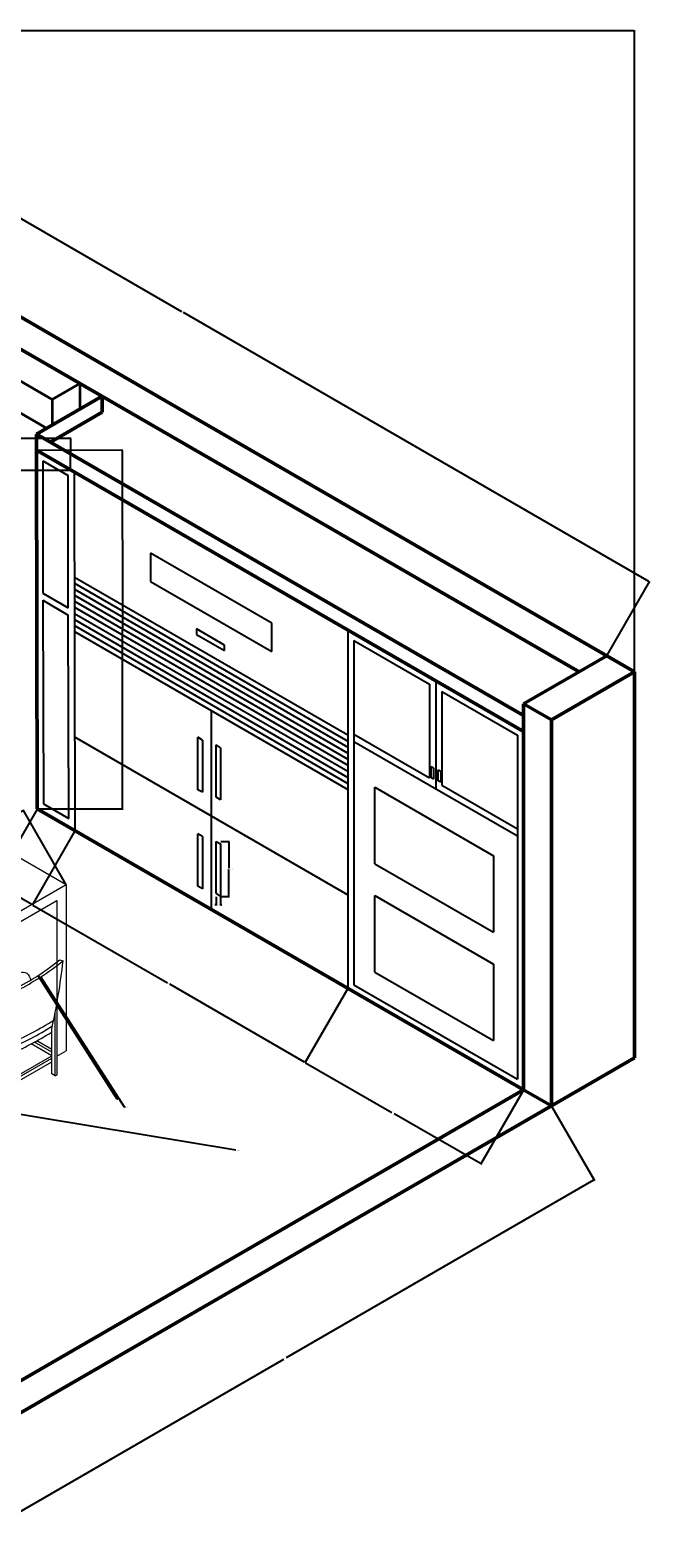
# Model space of a CAD drawing. Units: inches. Extents: x 4150 to 4636, y 2169 to 2592.
# Tile 8 of 8: x 4462 to 4636, y 2169 to 2592. Entities that reach past the tile are written whole.
import ezdxf

# ---------------------------------------------------------------- set-up
doc = ezdxf.new("R2010")
doc.units = ezdxf.units.IN
for name, color, linetype, lineweight in [('A-ANNO-DIMS', 2, 'Continuous', 18), ('A-EQPM', 6, 'Continuous', 25), ('A-FURN', 8, 'Continuous', 18), ('A-WALL', 7, 'Continuous', 50), ('S-BEAM', 1, 'Continuous', 35)]:
    doc.layers.add(name, color=color, linetype=linetype, lineweight=lineweight)
doc.styles.get("Standard").update_dxf_attribs({"font": 'arial.ttf'})
doc.dimstyles.get("Standard").update_dxf_attribs({"dimtxt": 0.18, "dimasz": 0.18, "dimexe": 0.18, "dimexo": 0.0625, "dimgap": 0.09, "dimtad": 0, "dimtih": 1, "dimtoh": 1, "dimdec": 4, "dimzin": 0, "dimdsep": 46, "dimtxsty": 'Standard', "dimcen": 0.09, "dimadec": 0, "dimazin": 0, "dimtfac": 1, "dimtdec": 4, "dimtofl": 0, "dimtmove": 0, "dimatfit": 3, "dimfxl": 1, "dimtolj": 1, "dimtzin": 0, "dimarcsym": 0})

# ---------------------------------------------------------------- blocks, each defined once
blk = doc.blocks.new('CHAIR')
for p, q in [((4460.61, 2323.17), (4462.07, 2322.64)), ((4458.4, 2267.81), (4458.4, 2298.32)), ((4459.26, 2268.31), (4459.26, 2302.96)), ((4419.13, 2296.33), (4418.72, 2294.28)), ((4434.61, 2281.77), (4418.72, 2294.28)), ((4418.72, 2294.28), (4418.72, 2263.74)), ((4435.02, 2283.82), (4419.13, 2296.33)), ((4419.58, 2264.24), (4419.58, 2293.6)), ((4421.31, 2292.24), (4421.31, 2265.24)), ((4436.24, 2283.27), (4435.02, 2283.82)), ((4456.67, 2279.13), (4448.46, 2283.88)), ((4456.67, 2280.34), (4449.53, 2284.46)), ((4456.67, 2268.81), (4456.67, 2290.03)), ((4421.31, 2274.06), (4434.6, 2281.73)), ((4421.31, 2272.85), (4434.31, 2280.36)), ((4421.31, 2271.17), (4433.9, 2278.43)), ((4435.2, 2254.23), (4435.2, 2278.19)), ((4436.06, 2254.73), (4436.06, 2282.33)), ((4436.06, 2265.55), (4456.67, 2277.45)), ((4456.67, 2277.45), (4446.94, 2283.07)), ((4433.46, 2267.05), (4421.31, 2274.06)), ((4433.46, 2265.84), (4421.31, 2272.85)), ((4433.46, 2264.15), (4421.31, 2271.17)), ((4433.46, 2255.23), (4433.46, 2276.44)), ((4436.06, 2264.34), (4456.67, 2276.24)), ((4436.06, 2262.66), (4456.67, 2274.56)), ((4418.72, 2263.74), (4419.58, 2264.24)), ((4419.58, 2264.24), (4421.31, 2265.24)), ((4458.4, 2267.81), (4456.67, 2268.81)), ((4458.4, 2267.81), (4459.26, 2268.31)), ((4435.2, 2254.23), (4433.46, 2255.23)), ((4435.2, 2254.23), (4436.06, 2254.73))]:
    blk.add_line(p, q)
for centre, radius, start, end in [((4387.22, 2413.69), 116.53, 296.3285, 309.03474), ((4384.96, 2418.26), 122.84, 296.66524, 308.88253), ((4169.51, 2354.34), 294.27, 347.37626, 353.81529), ((4146.35, 2340.95), 294.27, 347.33851, 353.81529), ((4147.53, 2340.19), 294.27, 347.83822, 353.81529), ((4388.03, 2399.21), 127.8, 292.07351, 302.67553), ((4388.03, 2401.62), 127.8, 292.16404, 302.99309), ((4387.7, 2396.31), 127.8, 292.23455, 302.66255)]:
    blk.add_arc(centre, radius, start, end)
blk.add_open_spline([(4419.13, 2296.33), (4419.73, 2299.09), (4421.22, 2306.03), (4435.02, 2305.47), (4437.67, 2317.36), (4445.4, 2317.24), (4446.24, 2314.8), (4446.7, 2313.47)], degree=3, knots=[0, 0, 0, 0, 7.695976, 19.302291, 31.993754, 35.157842, 38.967805, 38.967805, 38.967805, 38.967805])
blk = doc.blocks.new('FRIDGE-HANDLE')
for p, q in [((0, 0.81), (0, 15.46)), ((0, 15.46), (1.26, 14.74)), ((1.26, 14.74), (1.26, 0)), ((0, 0.81), (1.26, 0))]:
    blk.add_line(p, q)
blk = doc.blocks.new('*D24')
at = {"layer": 'A-ANNO-DIMS', "color": 0, "lineweight": -2, "transparency": 16777216}
for p, q in [((4515.27, 2364.38), (4517.7, 2364.38)), ((4517.52, 2364.2), (4517.52, 2356.83)), ((4517.52, 2349.1), (4517.52, 2356.46)), ((4515.27, 2348.92), (4517.7, 2348.92))]:
    blk.add_line(p, q, dxfattribs=at)
at = {"layer": 'A-ANNO-DIMS', "color": 0, "transparency": 16777216}
for points in [[(4517.49, 2364.2), (4517.55, 2364.2), (4517.52, 2364.38)], [(4517.49, 2349.1), (4517.55, 2349.1), (4517.52, 2348.92)]]:
    blk.add_solid(points, dxfattribs=at)
at = {"layer": 'Defpoints', "color": 0, "transparency": 16777216}
for p in [(4515.2, 2364.38), (4517.52, 2364.38), (4515.2, 2348.92)]:
    blk.add_point(p, dxfattribs=at)
at = {"layer": 'A-ANNO-DIMS', "color": 0, "transparency": 16777216, "insert": (4517.52, 2356.65), "char_height": 0.18, "attachment_point": 5}
blk.add_mtext('\\A1;FRIDGE HANDLE 15 TYP.', dxfattribs=at)
blk = doc.blocks.new('*D25')
at = {"layer": 'A-ANNO-DIMS', "color": 0, "lineweight": -2, "transparency": 16777216}
for p, q in [((4513.76, 2346.6), (4513.58, 2346.6)), ((4513.94, 2348.85), (4513.94, 2346.42)), ((4515.2, 2348.85), (4515.2, 2346.42)), ((4515.38, 2346.6), (4515.56, 2346.6))]:
    blk.add_line(p, q, dxfattribs=at)
at = {"layer": 'A-ANNO-DIMS', "color": 0, "transparency": 16777216}
for points in [[(4513.76, 2346.63), (4513.76, 2346.57), (4513.94, 2346.6)], [(4515.38, 2346.63), (4515.38, 2346.57), (4515.2, 2346.6)]]:
    blk.add_solid(points, dxfattribs=at)
at = {"layer": 'Defpoints', "color": 0, "transparency": 16777216}
for p in [(4513.94, 2348.92), (4515.2, 2348.92), (4515.2, 2346.6)]:
    blk.add_point(p, dxfattribs=at)
at = {"layer": 'A-ANNO-DIMS', "color": 0, "transparency": 16777216, "insert": (4514.57, 2346.6), "char_height": 0.18, "attachment_point": 5}
blk.add_mtext('\\A1;1 TYP.', dxfattribs=at)
blk = doc.blocks.new('*D36')
at = {"layer": 'A-ANNO-DIMS', "color": 0, "lineweight": -2, "transparency": 16777216}
for p, q in [((4174.28, 2460.03), (4174.28, 2592.15)), ((4174.46, 2591.97), (4402.51, 2591.97)), ((4631.36, 2591.97), (4403.31, 2591.97)), ((4631.54, 2412.03), (4631.54, 2592.15))]:
    blk.add_line(p, q, dxfattribs=at)
at = {"layer": 'A-ANNO-DIMS', "color": 0, "transparency": 16777216}
for points in [[(4174.46, 2592), (4174.46, 2591.94), (4174.28, 2591.97)], [(4631.36, 2592), (4631.36, 2591.94), (4631.54, 2591.97)]]:
    blk.add_solid(points, dxfattribs=at)
at = {"layer": 'Defpoints', "color": 0, "transparency": 16777216}
for p in [(4631.54, 2591.97), (4174.28, 2459.97), (4631.54, 2411.97)]:
    blk.add_point(p, dxfattribs=at)
at = {"layer": 'A-ANNO-DIMS', "color": 0, "transparency": 16777216, "insert": (4402.91, 2591.97), "char_height": 0.18, "attachment_point": 5}
blk.add_mtext('\\A1;457.3', dxfattribs=at)
blk = doc.blocks.new('*D39')
at = {"layer": 'A-ANNO-DIMS', "color": 0, "lineweight": -2, "transparency": 16777216}
for p, q in [((4608.19, 2290.05), (4620.25, 2269.16)), ((4620, 2269.23), (4533.6, 2219.34)), ((4446.56, 2169.09), (4532.97, 2218.98)), ((4434.43, 2189.73), (4446.49, 2168.84))]:
    blk.add_line(p, q, dxfattribs=at)
at = {"layer": 'A-ANNO-DIMS', "color": 0, "transparency": 16777216}
for points in [[(4619.99, 2269.25), (4620.02, 2269.2), (4620.16, 2269.32)], [(4446.54, 2169.11), (4446.57, 2169.06), (4446.4, 2169)]]:
    blk.add_solid(points, dxfattribs=at)
at = {"layer": 'Defpoints', "color": 0, "transparency": 16777216}
for p in [(4608.16, 2290.1), (4434.4, 2189.78), (4446.4, 2169)]:
    blk.add_point(p, dxfattribs=at)
at = {"layer": 'A-ANNO-DIMS', "color": 0, "transparency": 16777216, "insert": (4533.28, 2219.16), "char_height": 0.18, "attachment_point": 5}
blk.add_mtext('\\A1;200.64', dxfattribs=at)
blk = doc.blocks.new('*D43')
at = {"layer": 'A-ANNO-DIMS', "color": 0, "lineweight": -2, "transparency": 16777216}
for p, q in [((4361.37, 2568.02), (4373.43, 2588.91)), ((4373.5, 2588.66), (4504.26, 2513.17)), ((4635.59, 2437.34), (4504.83, 2512.83)), ((4623.78, 2416.52), (4635.84, 2437.41))]:
    blk.add_line(p, q, dxfattribs=at)
at = {"layer": 'A-ANNO-DIMS', "color": 0, "transparency": 16777216}
for points in [[(4373.51, 2588.69), (4373.48, 2588.63), (4373.34, 2588.75)], [(4635.61, 2437.37), (4635.58, 2437.31), (4635.75, 2437.25)]]:
    blk.add_solid(points, dxfattribs=at)
at = {"layer": 'Defpoints', "color": 0, "transparency": 16777216}
for p in [(4361.34, 2567.97), (4635.75, 2437.25), (4623.75, 2416.47)]:
    blk.add_point(p, dxfattribs=at)
at = {"layer": 'A-ANNO-DIMS', "color": 0, "transparency": 16777216, "insert": (4504.54, 2513), "char_height": 0.18, "attachment_point": 5}
blk.add_mtext('\\A1;303', dxfattribs=at)
blk = doc.blocks.new('*D46')
at = {"layer": 'A-ANNO-DIMS', "color": 0, "lineweight": -2, "transparency": 16777216}
for p, q in [((4449.11, 2477.6), (4473.23, 2477.6)), ((4473.05, 2477.42), (4473.05, 2473.29)), ((4473.05, 2468.78), (4473.05, 2472.92)), ((4449.11, 2468.6), (4473.23, 2468.6))]:
    blk.add_line(p, q, dxfattribs=at)
at = {"layer": 'A-ANNO-DIMS', "color": 0, "transparency": 16777216}
for points in [[(4473.02, 2477.42), (4473.08, 2477.42), (4473.05, 2477.6)], [(4473.02, 2468.78), (4473.08, 2468.78), (4473.05, 2468.6)]]:
    blk.add_solid(points, dxfattribs=at)
at = {"layer": 'Defpoints', "color": 0, "transparency": 16777216}
for p in [(4449.05, 2477.6), (4449.05, 2468.6), (4473.05, 2468.6)]:
    blk.add_point(p, dxfattribs=at)
at = {"layer": 'A-ANNO-DIMS', "color": 0, "transparency": 16777216, "insert": (4473.05, 2473.1), "char_height": 0.18, "attachment_point": 5}
blk.add_mtext('\\A1;9', dxfattribs=at)
blk = doc.blocks.new('*D62')
at = {"layer": 'A-ANNO-DIMS', "color": 0, "lineweight": -2, "transparency": 16777216}
for p, q in [((4463.66, 2373.46), (4451.6, 2352.57)), ((4474.29, 2367.32), (4462.23, 2346.43)), ((4451.85, 2352.64), (4456.69, 2349.84)), ((4462.17, 2346.68), (4457.32, 2349.48))]:
    blk.add_line(p, q, dxfattribs=at)
at = {"layer": 'A-ANNO-DIMS', "color": 0, "transparency": 16777216}
for points in [[(4451.86, 2352.66), (4451.83, 2352.61), (4451.69, 2352.73)], [(4462.18, 2346.7), (4462.15, 2346.65), (4462.32, 2346.59)]]:
    blk.add_solid(points, dxfattribs=at)
at = {"layer": 'Defpoints', "color": 0, "transparency": 16777216}
for p in [(4463.69, 2373.51), (4474.32, 2367.37), (4451.69, 2352.73)]:
    blk.add_point(p, dxfattribs=at)
at = {"layer": 'A-ANNO-DIMS', "color": 0, "transparency": 16777216, "insert": (4457.01, 2349.66), "char_height": 0.18, "attachment_point": 5}
blk.add_mtext('\\A1;12.278', dxfattribs=at)
blk = doc.blocks.new('*D63')
at = {"layer": 'A-ANNO-DIMS', "color": 0, "lineweight": -2, "transparency": 16777216}
for p, q in [((4474.29, 2367.32), (4462.23, 2346.43)), ((4462.48, 2346.5), (4500.33, 2324.65)), ((4538.8, 2302.43), (4500.96, 2324.28)), ((4550.93, 2323.07), (4538.87, 2302.19))]:
    blk.add_line(p, q, dxfattribs=at)
at = {"layer": 'A-ANNO-DIMS', "color": 0, "transparency": 16777216}
for points in [[(4462.49, 2346.52), (4462.46, 2346.47), (4462.32, 2346.59)], [(4538.82, 2302.46), (4538.79, 2302.41), (4538.96, 2302.34)]]:
    blk.add_solid(points, dxfattribs=at)
at = {"layer": 'Defpoints', "color": 0, "transparency": 16777216}
for p in [(4474.32, 2367.37), (4462.32, 2346.59), (4550.96, 2323.13)]:
    blk.add_point(p, dxfattribs=at)
at = {"layer": 'A-ANNO-DIMS', "color": 0, "transparency": 16777216, "insert": (4500.64, 2324.46), "char_height": 0.18, "attachment_point": 5}
blk.add_mtext('\\A1;88.5', dxfattribs=at)
blk = doc.blocks.new('*D64')
at = {"layer": 'A-ANNO-DIMS', "color": 0, "lineweight": -2, "transparency": 16777216}
for p, q in [((4550.93, 2323.07), (4538.87, 2302.19)), ((4539.11, 2302.25), (4563.35, 2288.26)), ((4600.33, 2294.55), (4588.27, 2273.66)), ((4588.21, 2273.91), (4563.98, 2287.9))]:
    blk.add_line(p, q, dxfattribs=at)
at = {"layer": 'A-ANNO-DIMS', "color": 0, "transparency": 16777216}
for points in [[(4539.13, 2302.28), (4539.1, 2302.23), (4538.96, 2302.34)], [(4588.22, 2273.93), (4588.19, 2273.88), (4588.36, 2273.82)]]:
    blk.add_solid(points, dxfattribs=at)
at = {"layer": 'Defpoints', "color": 0, "transparency": 16777216}
for p in [(4550.96, 2323.13), (4538.96, 2302.34), (4600.36, 2294.6)]:
    blk.add_point(p, dxfattribs=at)
at = {"layer": 'A-ANNO-DIMS', "color": 0, "transparency": 16777216, "insert": (4563.66, 2288.08), "char_height": 0.18, "attachment_point": 5}
blk.add_mtext('\\A1;57.05', dxfattribs=at)
blk = doc.blocks.new('*D65')
at = {"layer": 'A-ANNO-DIMS', "color": 0, "lineweight": -2, "transparency": 16777216}
for p, q in [((4463.58, 2474.23), (4487.7, 2474.28)), ((4487.52, 2474.1), (4487.6, 2424.1)), ((4487.69, 2373.73), (4487.6, 2423.73)), ((4463.75, 2373.51), (4487.87, 2373.55))]:
    blk.add_line(p, q, dxfattribs=at)
at = {"layer": 'A-ANNO-DIMS', "color": 0, "transparency": 16777216}
for points in [[(4487.55, 2474.1), (4487.49, 2474.1), (4487.52, 2474.28)], [(4487.72, 2373.73), (4487.66, 2373.73), (4487.69, 2373.55)]]:
    blk.add_solid(points, dxfattribs=at)
at = {"layer": 'Defpoints', "color": 0, "transparency": 16777216}
for p in [(4463.52, 2474.23), (4463.69, 2373.51), (4487.69, 2373.55)]:
    blk.add_point(p, dxfattribs=at)
at = {"layer": 'A-ANNO-DIMS', "color": 0, "transparency": 16777216, "insert": (4487.6, 2423.91), "char_height": 0.18, "attachment_point": 5}
blk.add_mtext('\\A1;100.72', dxfattribs=at)
blk = doc.blocks.new('*D67')
at = {"layer": 'A-ANNO-DIMS', "color": 0, "lineweight": -2, "transparency": 16777216}
for p, q in [((4459.63, 2373), (4418.44, 2349.22)), ((4471.75, 2352.36), (4459.7, 2373.25)), ((4376.8, 2325.18), (4418, 2348.96)), ((4388.62, 2304.36), (4376.56, 2325.25))]:
    blk.add_line(p, q, dxfattribs=at)
at = {"layer": 'A-ANNO-DIMS', "color": 0, "transparency": 16777216}
for points in [[(4459.62, 2373.03), (4459.65, 2372.98), (4459.79, 2373.09)], [(4376.79, 2325.21), (4376.82, 2325.16), (4376.65, 2325.09)]]:
    blk.add_solid(points, dxfattribs=at)
at = {"layer": 'Defpoints', "color": 0, "transparency": 16777216}
for p in [(4459.79, 2373.09), (4471.79, 2352.31), (4388.65, 2304.31)]:
    blk.add_point(p, dxfattribs=at)
at = {"layer": 'A-ANNO-DIMS', "color": 0, "transparency": 16777216, "insert": (4418.22, 2349.09), "char_height": 0.18, "attachment_point": 5}
blk.add_mtext('\\A1;96', dxfattribs=at)
blk = doc.blocks.new('*D75')
at = {"layer": 'A-ANNO-DIMS', "color": 0, "lineweight": -2, "transparency": 16777216}
for p, q in [((4245.64, 2323.02), (4245.82, 2323.02)), ((4245.73, 2322.93), (4245.73, 2323.11)), ((4519.53, 2277.67), (4417.03, 2294.65))]:
    blk.add_line(p, q, dxfattribs=at)
at = {"layer": 'A-ANNO-DIMS', "color": 0, "transparency": 16777216}
blk.add_solid([(4417.03, 2294.68), (4417.02, 2294.62), (4416.85, 2294.68)], dxfattribs=at)
at = {"layer": 'Defpoints', "color": 0, "transparency": 16777216}
for p in [(4245.73, 2323.02), (4416.85, 2294.68)]:
    blk.add_point(p, dxfattribs=at)
at = {"layer": 'A-ANNO-DIMS', "color": 0, "transparency": 16777216, "insert": (4520.08, 2277.67), "char_height": 0.18, "attachment_point": 5}
blk.add_mtext('\\A1;R173.46', dxfattribs=at)
blk = doc.blocks.new('*D77')
at = {"layer": 'A-ANNO-DIMS', "color": 0, "lineweight": -2, "transparency": 16777216}
for p, q in [((4425.39, 2387.21), (4425.57, 2387.21)), ((4425.48, 2387.12), (4425.48, 2387.3)), ((4488.19, 2289.8), (4464.77, 2326.18)), ((4488.37, 2289.8), (4488.19, 2289.8))]:
    blk.add_line(p, q, dxfattribs=at)
at = {"layer": 'A-ANNO-DIMS', "color": 0, "transparency": 16777216}
blk.add_solid([(4464.8, 2326.19), (4464.75, 2326.16), (4464.68, 2326.33)], dxfattribs=at)
at = {"layer": 'Defpoints', "color": 0, "transparency": 16777216}
for p in [(4425.48, 2387.21), (4464.68, 2326.33)]:
    blk.add_point(p, dxfattribs=at)
at = {"layer": 'A-ANNO-DIMS', "color": 0, "transparency": 16777216, "insert": (4488.84, 2289.8), "char_height": 0.18, "attachment_point": 5}
blk.add_mtext('\\A1;R72.41', dxfattribs=at)
blk = doc.blocks.new('*D78')
at = {"layer": 'A-ANNO-DIMS', "color": 0, "lineweight": -2, "transparency": 16777216}
for p, q in [((4426.72, 2384.51), (4426.9, 2384.51)), ((4426.81, 2384.42), (4426.81, 2384.6)), ((4486.16, 2292.01), (4464, 2326.55)), ((4486.34, 2292.01), (4486.16, 2292.01))]:
    blk.add_line(p, q, dxfattribs=at)
at = {"layer": 'A-ANNO-DIMS', "color": 0, "transparency": 16777216}
blk.add_solid([(4464.03, 2326.56), (4463.98, 2326.53), (4463.9, 2326.7)], dxfattribs=at)
at = {"layer": 'Defpoints', "color": 0, "transparency": 16777216}
for p in [(4426.81, 2384.51), (4463.9, 2326.7)]:
    blk.add_point(p, dxfattribs=at)
at = {"layer": 'A-ANNO-DIMS', "color": 0, "transparency": 16777216, "insert": (4486.82, 2292.01), "char_height": 0.18, "attachment_point": 5}
blk.add_mtext('\\A1;R68.69', dxfattribs=at)

msp = doc.modelspace()

# ---------------------------------------------------------------- linework, layer by layer
at = {"layer": 'A-EQPM'}
for p, q in [((4465.2501, 2471.2343), (4465.2501, 2434.0676)), ((4465.2501, 2471.2343), (4472.4192, 2467.0952)), ((4474.3231, 2367.372), (4474.1513, 2468.0952)), ((4474.1513, 2468.0952), (4550.9589, 2423.7503)), ((4472.4192, 2429.9285), (4472.4192, 2467.0952)), ((4529.5665, 2425.6516), (4495.5437, 2445.2946)), ((4495.5437, 2445.2946), (4495.5437, 2437.3101)), ((4474.1513, 2438.6014), (4550.9589, 2394.2565)), ((4465.2501, 2434.0676), (4472.4192, 2429.9285)), ((4474.1513, 2436.9011), (4550.9589, 2392.5562)), ((4474.1513, 2435.2008), (4550.9589, 2390.8559)), ((4495.5437, 2437.3101), (4529.5665, 2417.667)), ((4465.2501, 2432.0676), (4472.4192, 2427.9285)), ((4465.2501, 2432.0676), (4465.4213, 2374.9185)), ((4474.1513, 2433.5006), (4550.9589, 2389.1557)), ((4474.1513, 2431.8003), (4550.9589, 2387.4554)), ((4474.1513, 2430.1), (4550.9589, 2385.7551)), ((4472.5904, 2370.7794), (4472.4192, 2427.9285)), ((4474.1513, 2428.3997), (4550.9589, 2384.0548)), ((4474.1513, 2426.6995), (4550.9589, 2382.3545)), ((4529.5665, 2417.667), (4529.5665, 2425.6516)), ((4474.1513, 2424.9992), (4550.9589, 2380.6543)), ((4474.1513, 2423.2989), (4550.9589, 2378.954)), ((4516.3444, 2419.5139), (4508.4817, 2424.0535)), ((4508.4817, 2424.0535), (4508.4817, 2422.4819)), ((4508.4817, 2422.4819), (4516.3444, 2417.9424)), ((4550.9589, 2423.7503), (4550.9589, 2323.1264)), ((4516.3444, 2417.9424), (4516.3444, 2419.5139)), ((4552.691, 2420.7503), (4552.691, 2324.1264)), ((4552.691, 2420.7503), (4573.9296, 2408.4882)), ((4575.6617, 2409.4882), (4575.6617, 2379.1849)), ((4573.9296, 2408.4882), (4573.9296, 2382.1849)), ((4577.3937, 2406.4882), (4577.3937, 2380.1849)), ((4577.3937, 2406.4882), (4598.6324, 2394.226)), ((4512.5551, 2401.1264), (4512.5551, 2345.2988)), ((4474.1513, 2393.699), (4550.9589, 2349.3541)), ((4552.691, 2394.4471), (4573.9296, 2382.1849)), ((4552.691, 2392.4471), (4598.6324, 2365.9227)), ((4598.6324, 2394.226), (4598.6324, 2297.602)), ((4574.3544, 2382.2326), (4574.3544, 2385.3699)), ((4574.3544, 2385.3699), (4575.03, 2384.9798)), ((4575.03, 2384.9798), (4575.03, 2381.8426)), ((4576.3824, 2381.3704), (4576.3824, 2384.5077)), ((4576.3824, 2384.5077), (4577.0579, 2384.1177)), ((4577.0579, 2384.1177), (4577.0579, 2380.9804)), ((4558.5181, 2358.0987), (4558.5181, 2379.5967)), ((4558.5181, 2379.5967), (4591.8494, 2360.3529)), ((4575.03, 2381.8426), (4574.3544, 2382.2326)), ((4577.0579, 2380.9804), (4576.3824, 2381.3704)), ((4577.3937, 2380.1849), (4598.6324, 2367.9227)), ((4465.4213, 2374.9185), (4472.5904, 2370.7794)), ((4463.513, 2373.6133), (4474.1462, 2367.4742)), ((4558.5181, 2358.0987), (4591.8494, 2338.8549)), ((4591.8494, 2360.3529), (4591.8494, 2338.8549)), ((4558.5181, 2327.6892), (4558.5181, 2349.1873)), ((4558.5181, 2349.1873), (4591.8494, 2329.9434)), ((4591.8494, 2329.9434), (4591.8494, 2308.4454)), ((4552.691, 2324.1264), (4598.6324, 2297.602)), ((4558.5181, 2327.6892), (4591.8494, 2308.4454)), ((4552.691, 2322.1264), (4598.6324, 2295.602))]:
    msp.add_line(p, q, dxfattribs=at)
at = {"layer": 'A-FURN'}
for p, q in [((4432.8151, 2374.8064), (4471.7862, 2352.3064)), ((4388.6478, 2304.3064), (4471.7862, 2352.3064)), ((4471.7862, 2352.3064), (4471.7862, 2305.5436)), ((4391.2458, 2302.8064), (4469.1881, 2347.8064)), ((4469.1881, 2347.8064), (4469.1881, 2304.0436)), ((4469.1881, 2304.0436), (4471.7862, 2305.5436))]:
    msp.add_line(p, q, dxfattribs=at)
at = {"layer": 'A-WALL'}
for p, q in [((4361.3415, 2567.9652), (4506.8337, 2483.9652)), ((4361.3415, 2558.9652), (4615.9529, 2411.9652)), ((4463.5181, 2478.7343), (4481.9117, 2489.3539)), ((4481.9117, 2489.3539), (4481.9117, 2484.8539)), ((4481.9117, 2484.8539), (4467.4152, 2476.4843)), ((4506.8337, 2483.9652), (4631.5414, 2411.9652)), ((4463.5181, 2474.2343), (4463.5181, 2478.7343)), ((4463.5181, 2478.7343), (4600.3645, 2399.726)), ((4463.5181, 2474.2343), (4600.3645, 2395.226)), ((4463.5181, 2474.2343), (4463.6899, 2373.5111)), ((4552.691, 2422.7503), (4600.3645, 2395.226)), ((4600.3645, 2402.9652), (4623.7472, 2416.4652)), ((4631.5414, 2411.9652), (4608.1587, 2398.4652)), ((4631.5414, 2411.9652), (4631.5414, 2303.602)), ((4608.1587, 2398.4652), (4600.3645, 2402.9652)), ((4600.3645, 2402.9652), (4600.3645, 2294.602)), ((4600.3645, 2402.9652), (4608.1587, 2398.4652)), ((4608.1587, 2398.4652), (4608.1587, 2290.102)), ((4600.3645, 2294.602), (4463.6899, 2373.5111)), ((4434.4021, 2189.7836), (4631.5414, 2303.602)), ((4434.204, 2198.6692), (4600.3645, 2294.602)), ((4608.1587, 2290.102), (4600.3645, 2294.602))]:
    msp.add_line(p, q, dxfattribs=at)
at = {"layer": 'S-BEAM'}
for p, q in [((4353.5472, 2554.4652), (4467.8626, 2488.4652)), ((4353.5472, 2545.4652), (4466.3233, 2480.3539)), ((4475.6568, 2492.9652), (4467.8626, 2488.4652)), ((4475.6568, 2492.9652), (4475.6568, 2485.7426)), ((4467.8626, 2488.4652), (4467.8626, 2481.2426))]:
    msp.add_line(p, q, dxfattribs=at)

# ---------------------------------------------------------------- block references
at = {"layer": 'A-EQPM', "rotation": 180.0247430787337}
for p in [(4510.1055, 2393.6222), (4515.1991, 2391.4957), (4510.1055, 2366.5481)]:
    msp.add_blockref('FRIDGE-HANDLE', p, dxfattribs=at)
at = {"layer": 'A-EQPM'}
msp.add_blockref('FRIDGE-HANDLE', (4513.945, 2348.915), dxfattribs=at)
at = {"layer": 'A-FURN', "xscale": 0.5894434727893052, "yscale": 0.5894434727893052, "zscale": 0.5894434727893052}
msp.add_blockref('CHAIR', (1840.7944, 961.7822), dxfattribs=at)

# ---------------------------------------------------------------- dimensions: what is measured, and where the dimension line sits
at = {"layer": 'A-ANNO-DIMS'}
dim = msp.add_linear_dim(base=(4631.5414, 2591.9652), p1=(4174.28, 2459.9652), p2=(4631.5414, 2411.9652), dimstyle='Standard', override={"dimdec": 1, "dimlfac": 1, "dimrnd": 0, "dimzin": 0, "dimdsep": 46, "dimlunit": 2}, dxfattribs=at)
dim.commit()
dim.dimension.update_dxf_attribs({"geometry": '*D36', "text_midpoint": (4402.9107, 2591.9652)})
for base, p1, p2, angle, override, picture, middle in [((4635.7472, 2437.2498), (4361.3415, 2567.9652), (4623.7472, 2416.4652), 330, {"dimdec": 0, "dimlfac": 1, "dimrnd": 0, "dimzin": 0, "dimdsep": 46, "dimlunit": 2}, '*D43', (4504.5443, 2512.9998)), ((4473.0511, 2468.6043), (4449.0511, 2477.6043), (4449.0511, 2468.6043), 270, {"dimdec": 0, "dimlfac": 1, "dimrnd": 0, "dimzin": 0, "dimdsep": 46, "dimlunit": 2}, '*D46', (4473.0511, 2473.1043)), ((4487.6899, 2373.5521), (4463.5181, 2474.2343), (4463.6899, 2373.5111), 270.09777, {"dimdec": 2, "dimlfac": 1, "dimrnd": 0, "dimzin": 0, "dimdsep": 46, "dimlunit": 2}, '*D65', (4487.604, 2423.9137)), ((4459.7862, 2373.091), (4388.6478, 2304.3064), (4471.7862, 2352.3064), 30, {"dimdec": 0, "dimlfac": 1, "dimrnd": 0, "dimzin": 0, "dimdsep": 46, "dimlunit": 2}, '*D67', (4418.217, 2349.091)), ((4451.6899, 2352.7265), (4474.3231, 2367.372), (4463.6899, 2373.5111), 150, {"dimdec": 3, "dimlfac": 1, "dimrnd": 0, "dimzin": 0, "dimdsep": 46, "dimlunit": 2}, '*D62', (4457.0065, 2349.657)), ((4462.3231, 2346.5874), (4550.9589, 2323.1264), (4474.3231, 2367.372), 150, {"dimdec": 1, "dimlfac": 1, "dimrnd": 0, "dimzin": 0, "dimdsep": 46, "dimlunit": 2}, '*D63', (4500.641, 2324.4646)), ((4538.9589, 2302.3418), (4600.3645, 2294.602), (4550.9589, 2323.1264), 150, {"dimdec": 2, "dimlfac": 1, "dimrnd": 0, "dimzin": 0, "dimdsep": 46, "dimlunit": 2}, '*D64', (4563.6617, 2288.0796)), ((4446.4021, 2168.999), (4608.1587, 2290.102), (4434.4021, 2189.7836), 210, {"dimdec": 2, "dimlfac": 1, "dimrnd": 0, "dimzin": 0, "dimdsep": 46, "dimlunit": 2}, '*D39', (4533.2804, 2219.1582))]:
    dim = msp.add_linear_dim(base=base, p1=p1, p2=p2, angle=angle, dimstyle='Standard', override=override, dxfattribs=at)
    dim.commit()
    dim.dimension.update_dxf_attribs({"geometry": picture, "text_midpoint": middle})
for center, mpoint, picture, middle in [((4425.4794, 2387.2104), (4464.6759, 2326.3282), '*D77', (4488.8362, 2289.7989)), ((4426.8142, 2384.5135), (4463.904, 2326.699), '*D78', (4486.8179, 2292.0103)), ((4245.7269, 2323.0174), (4416.8518, 2294.675), '*D75', (4519.5268, 2277.6696))]:
    dim = msp.add_radius_dim(center=center, mpoint=mpoint, dimstyle='Standard', override={"dimdec": 2, "dimlfac": 1, "dimrnd": 0, "dimzin": 0, "dimdsep": 46, "dimlunit": 2}, dxfattribs=at)
    dim.commit()
    dim.dimension.update_dxf_attribs({"geometry": picture, "text_midpoint": middle, "dimtype": 164})
dim = msp.add_linear_dim(base=(4517.5226, 2364.38), p1=(4515.2029, 2348.9151), p2=(4515.2029, 2364.38), angle=90, text='FRIDGE HANDLE <> TYP.', dimstyle='Standard', override={"dimdec": 0, "dimlfac": 1, "dimrnd": 0, "dimzin": 0, "dimdsep": 46, "dimlunit": 2}, dxfattribs=at)
dim.commit()
dim.dimension.update_dxf_attribs({"geometry": '*D24', "text_midpoint": (4517.5226, 2356.6475)})
dim = msp.add_linear_dim(base=(4515.2029, 2346.5954), p1=(4513.9445, 2348.9151), p2=(4515.2029, 2348.9151), text='<> TYP.', dimstyle='Standard', override={"dimdec": 0, "dimlfac": 1, "dimrnd": 0, "dimzin": 0, "dimdsep": 46, "dimlunit": 2}, dxfattribs=at)
dim.commit()
dim.dimension.update_dxf_attribs({"geometry": '*D25', "text_midpoint": (4514.5737, 2346.5954)})

doc.saveas('drawing.dxf')
